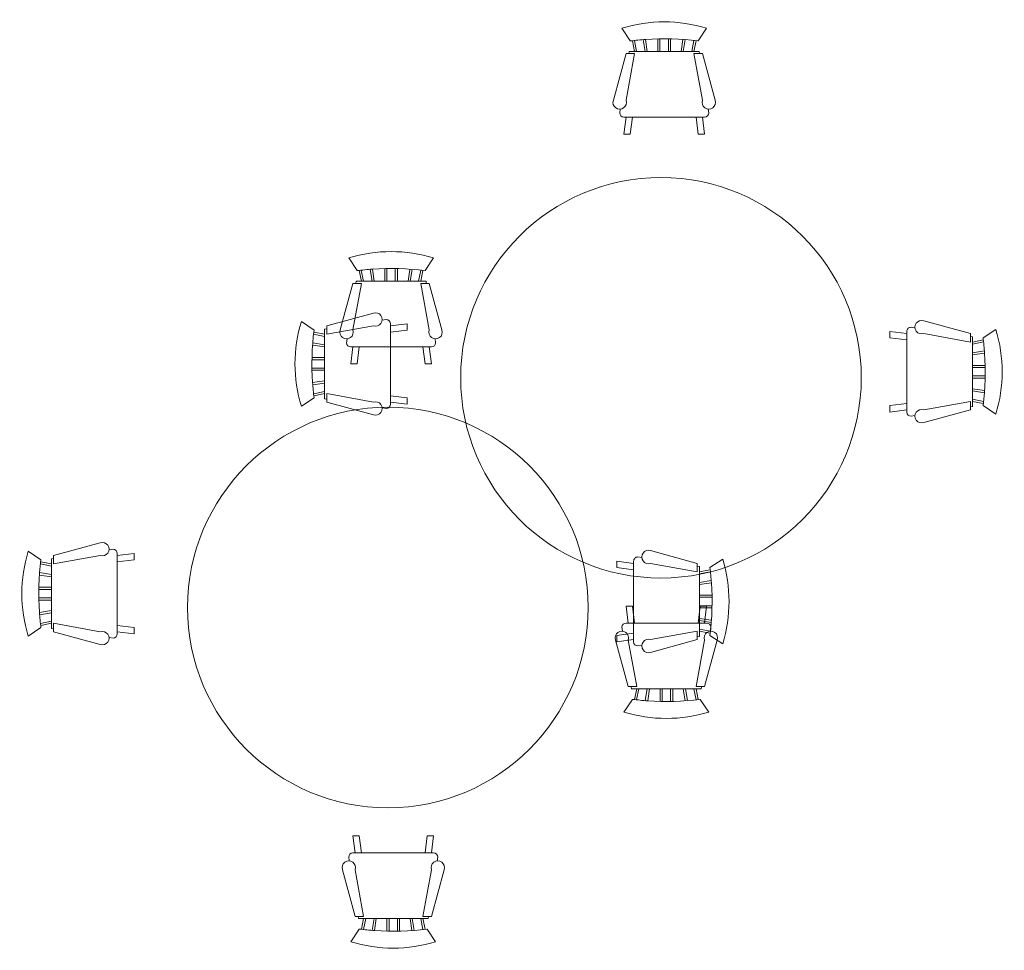
# Model space of a CAD drawing. Units: inches. Extents: x 2165 to 6441, y 2023 to 4425.
# Tile 4 of 4: x 6331 to 6441, y 4321 to 4425. Entities that reach past the tile are written whole.
import ezdxf

# ---------------------------------------------------------------- set-up
doc = ezdxf.new("R2010")
doc.units = ezdxf.units.IN
doc.layers.add('furniture', color=9, linetype='Continuous', lineweight=18)

# ---------------------------------------------------------------- blocks, each defined once
blk = doc.blocks.new('Chair - Rocking')
for p, q in [((-8, -4.5), (-10, -1.5)), ((8, -4.5), (10, -1.5)), ((-7.5, -4.5), (-7, -7)), ((-6.5, -7), (-7.02225, -4.43)), ((-4.5, -7), (-4.96674, -4.19951)), ((-4, -7), (-4.40532, -4.16272)), ((-1.5, -4.05012), (-1.5, -7)), ((-1, -7), (-1, -4.05012)), ((1, -7), (1, -4.04655)), ((1.5, -4.05012), (1.5, -7)), ((4, -7), (4.40187, -4.18694)), ((4.5, -7), (4.96761, -4.19437)), ((6.5, -7), (7, -4.4057)), ((7.5, -4.5), (7, -7)), ((-9, -7.5), (-12, -18.49999)), ((-7, -7.5), (-9, -7.5)), ((-9, -18.49999), (-7, -7.5)), ((-8.23428, -6.99939), (-8.3093, -7.47958)), ((-8.23041, -7), (8.23915, -7)), ((7, -7.5), (9, -7.5)), ((9, -18.49999), (7, -7.5)), ((8.31071, -7.48854), (8.23449, -7.00073)), ((9, -7.5), (12, -18.49999)), ((-10.36644, -20.64523), (-10.5, -21.49999)), ((10.5, -21.49999), (10.3575, -20.58798)), ((-9, -22.49999), (-9.5, -26.49999)), ((0, -22.49999), (-9.5, -22.49999)), ((-8, -26.49999), (-7.5, -22.49999)), ((0, -22.49999), (9.5, -22.49999)), ((8, -26.49999), (7.5, -22.49999)), ((9, -22.49999), (9.5, -26.49999)), ((-9.5, -26.49999), (-8, -26.49999)), ((9.5, -26.49999), (8, -26.49999))]:
    blk.add_line(p, q)
for centre, radius, start, end in [((0, -34.08333), 34.08333, 72.93847, 107.0615), ((0, -68.25004), 64.25, 93.92211, 97.15267), ((0, -68.25004), 64.25, 82.84733, 93.92211), ((-10.5, -18.99999), 1.58114, 161.5651, 18.43495), ((10.5, -18.99999), 1.58114, 161.5651, 18.43495), ((-9.5, -21.49999), 1, 180, 270), ((9.5, -21.49999), 1, 270, 0)]:
    blk.add_arc(centre, radius, start, end)
blk = doc.blocks.new('DINING TABLE (1)')
at = {"layer": 'furniture'}
blk.add_circle((3620.82, 1975.86), 22.28, dxfattribs=at)
at = {"layer": 'furniture', "xscale": 0.4715696020478906, "yscale": 0.4715696020478906, "zscale": 0.4715696020478906}
blk.add_blockref('Chair - Rocking', (3621.18, 2015.46), dxfattribs=at)
at = {"layer": 'furniture', "yscale": 0.4715696020478906, "zscale": 0.4715696020478906}
for p, xscale, rotation in [((3580.11, 1977.4), 0.4715696020478906, 90), ((3658.77, 1976.53), 0.4715696020478906, 270), ((3621.42, 1937.96), -0.4715696020478906, 180)]:
    blk.add_blockref('Chair - Rocking', p, dxfattribs=dict(at, xscale=xscale, rotation=rotation))

msp = doc.modelspace()

# ---------------------------------------------------------------- block references
at = {"layer": 'furniture'}
for p in [(2781.89, 2409.21), (2751.51, 2383.65)]:
    msp.add_blockref('DINING TABLE (1)', p, dxfattribs=at)

doc.saveas('drawing.dxf')
